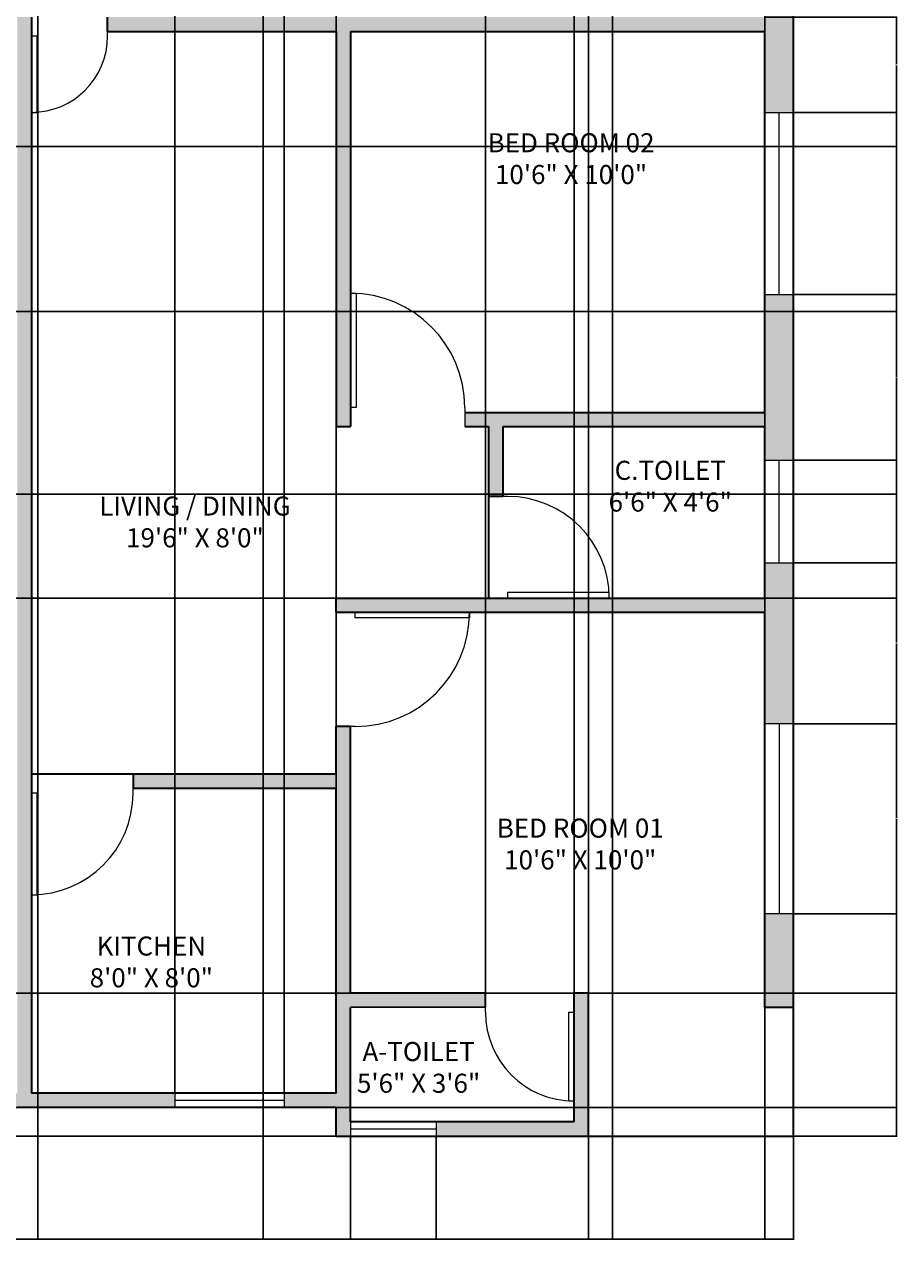
# Model space of a CAD drawing. Units: inches. Extents: x 2510 to 3056, y 673 to 1386.
# Tile 2 of 4: x 2781 to 3056, y 673 to 1056. Entities that reach past the tile are written whole.
import ezdxf

# ---------------------------------------------------------------- set-up
doc = ezdxf.new("R2010")
doc.units = ezdxf.units.IN
for name, color, linetype, lineweight in [('A-ANNO-DIMS', 2, 'Continuous', 18), ('A-AREA-IDEN', 7, 'Continuous', 18), ('A-DOOR', 3, 'Continuous', 18), ('A-GLAZ', 4, 'Continuous', 18), ('A-WALL', 7, 'Continuous', 35), ('A-WALL-PATT', 252, 'Continuous', 13)]:
    doc.layers.add(name, color=color, linetype=linetype, lineweight=lineweight)
doc.styles.get("Standard").update_dxf_attribs({"font": 'arial.ttf'})
doc.dimstyles.get("Standard").update_dxf_attribs({"dimtxt": 0.18, "dimasz": 0.18, "dimexe": 0.18, "dimexo": 0.0625, "dimgap": 0.09, "dimtad": 0, "dimtih": 1, "dimtoh": 1, "dimdec": 4, "dimzin": 0, "dimdsep": 46, "dimtxsty": 'Standard', "dimcen": 0.09, "dimadec": 0, "dimazin": 0, "dimtfac": 1, "dimtdec": 4, "dimtofl": 0, "dimtmove": 0, "dimatfit": 3, "dimfxl": 1, "dimtolj": 1, "dimtzin": 0, "dimarcsym": 0})

# ---------------------------------------------------------------- blocks, each defined once
blk = doc.blocks.new('*U6')
for p, q in [((0, 0), (0, -6)), ((36, 0), (36, -6))]:
    blk.add_line(p, q)
blk.add_lwpolyline([(0, 0), (0, 36), (1.75, 36), (1.75, 0)], close=True)
blk.add_arc((0, 0), 36, 0, 90)
blk = doc.blocks.new('*U7')
for p, q in [((0, 0), (0, 6)), ((24, 0), (24, 6))]:
    blk.add_line(p, q)
blk.add_lwpolyline([(0, 0), (0, -24), (1.75, -24), (1.75, 0)], close=True)
blk.add_arc((0, 0), 24, 270, 0)
blk = doc.blocks.new('*U5')
for p, q in [((0, 0), (0, 6)), ((32, 0), (32, 6))]:
    blk.add_line(p, q)
blk.add_lwpolyline([(0, 0), (0, -32), (1.75, -32), (1.75, 0)], close=True)
blk.add_arc((0, 0), 32, 270, 0)
blk = doc.blocks.new('*U11')
for p, q in [((-36, 0), (-36, 6)), ((0, 0), (0, 6))]:
    blk.add_line(p, q)
blk.add_lwpolyline([(0, 0), (0, -36), (-1.75, -36), (-1.75, 0)], close=True)
blk.add_arc((0, 0), 36, 180, 270)
blk = doc.blocks.new('*U10')
for p, q in [((-28, 0), (-28, 6)), ((0, 0), (0, 6))]:
    blk.add_line(p, q)
blk.add_lwpolyline([(0, 0), (0, -28), (-1.75, -28), (-1.75, 0)], close=True)
blk.add_arc((0, 0), 28, 180, 270)
blk = doc.blocks.new('*D13')
at = {"layer": 'A-ANNO-DIMS', "color": 0, "lineweight": -2, "transparency": 16777216}
for p, q in [((2543.19, 705.52), (2543.19, 672.93)), ((3023.19, 705.52), (3023.19, 672.93)), ((2543.37, 673.11), (2782.9, 673.11)), ((3023.01, 673.11), (2783.48, 673.11))]:
    blk.add_line(p, q, dxfattribs=at)
at = {"layer": 'A-ANNO-DIMS', "color": 0, "transparency": 16777216}
for points in [[(2543.37, 673.14), (2543.37, 673.08), (2543.19, 673.11)], [(3023.01, 673.14), (3023.01, 673.08), (3023.19, 673.11)]]:
    blk.add_solid(points, dxfattribs=at)
at = {"layer": 'Defpoints', "color": 0, "transparency": 16777216}
for p in [(2543.19, 705.59), (3023.19, 705.59), (3023.19, 673.11)]:
    blk.add_point(p, dxfattribs=at)
at = {"layer": 'A-ANNO-DIMS', "color": 0, "transparency": 16777216, "insert": (2783.19, 673.11), "char_height": 0.18, "attachment_point": 5}
blk.add_mtext('\\A1;480', dxfattribs=at)
blk = doc.blocks.new('*D22')
at = {"layer": 'A-ANNO-DIMS', "color": 0, "lineweight": -2, "transparency": 16777216}
for p, q in [((3023.25, 775.63), (3055.85, 775.63)), ((3055.67, 775.45), (3055.67, 740.79)), ((3055.67, 705.77), (3055.67, 740.43)), ((3023.25, 705.59), (3055.85, 705.59))]:
    blk.add_line(p, q, dxfattribs=at)
at = {"layer": 'A-ANNO-DIMS', "color": 0, "transparency": 16777216}
for points in [[(3055.64, 775.45), (3055.7, 775.45), (3055.67, 775.63)], [(3055.64, 705.77), (3055.7, 705.77), (3055.67, 705.59)]]:
    blk.add_solid(points, dxfattribs=at)
at = {"layer": 'Defpoints', "color": 0, "transparency": 16777216}
for p in [(3023.19, 775.63), (3055.67, 775.63), (3023.19, 705.59)]:
    blk.add_point(p, dxfattribs=at)
at = {"layer": 'A-ANNO-DIMS', "color": 0, "transparency": 16777216, "insert": (3055.67, 740.61), "char_height": 0.18, "attachment_point": 5}
blk.add_mtext('\\A1;70.04', dxfattribs=at)
blk = doc.blocks.new('*D23')
at = {"layer": 'A-ANNO-DIMS', "color": 0, "lineweight": -2, "transparency": 16777216}
for p, q in [((3023.25, 835.48), (3055.85, 835.48)), ((3055.67, 835.3), (3055.67, 805.74)), ((3055.67, 775.81), (3055.67, 805.37)), ((3023.25, 775.63), (3055.85, 775.63))]:
    blk.add_line(p, q, dxfattribs=at)
at = {"layer": 'A-ANNO-DIMS', "color": 0, "transparency": 16777216}
for points in [[(3055.64, 835.3), (3055.7, 835.3), (3055.67, 835.48)], [(3055.64, 775.81), (3055.7, 775.81), (3055.67, 775.63)]]:
    blk.add_solid(points, dxfattribs=at)
at = {"layer": 'Defpoints', "color": 0, "transparency": 16777216}
for p in [(3023.19, 835.48), (3055.67, 835.48), (3023.19, 775.63)]:
    blk.add_point(p, dxfattribs=at)
at = {"layer": 'A-ANNO-DIMS', "color": 0, "transparency": 16777216, "insert": (3055.67, 805.56), "char_height": 0.18, "attachment_point": 5}
blk.add_mtext('\\A1;59.85', dxfattribs=at)
blk = doc.blocks.new('*D24')
at = {"layer": 'A-ANNO-DIMS', "color": 0, "lineweight": -2, "transparency": 16777216}
for p, q in [((3023.25, 886.22), (3055.85, 886.22)), ((3055.67, 886.04), (3055.67, 861.03)), ((3055.67, 835.66), (3055.67, 860.67)), ((3023.25, 835.48), (3055.85, 835.48))]:
    blk.add_line(p, q, dxfattribs=at)
at = {"layer": 'A-ANNO-DIMS', "color": 0, "transparency": 16777216}
for points in [[(3055.64, 886.04), (3055.7, 886.04), (3055.67, 886.22)], [(3055.64, 835.66), (3055.7, 835.66), (3055.67, 835.48)]]:
    blk.add_solid(points, dxfattribs=at)
at = {"layer": 'Defpoints', "color": 0, "transparency": 16777216}
for p in [(3023.19, 886.22), (3055.67, 886.22), (3023.19, 835.48)]:
    blk.add_point(p, dxfattribs=at)
at = {"layer": 'A-ANNO-DIMS', "color": 0, "transparency": 16777216, "insert": (3055.67, 860.85), "char_height": 0.18, "attachment_point": 5}
blk.add_mtext('\\A1;50.74', dxfattribs=at)
blk = doc.blocks.new('*D25')
at = {"layer": 'A-ANNO-DIMS', "color": 0, "lineweight": -2, "transparency": 16777216}
for p, q in [((3023.25, 918.54), (3055.85, 918.54)), ((3055.67, 918.36), (3055.67, 902.56)), ((3055.67, 886.4), (3055.67, 902.2)), ((3023.25, 886.22), (3055.85, 886.22))]:
    blk.add_line(p, q, dxfattribs=at)
at = {"layer": 'A-ANNO-DIMS', "color": 0, "transparency": 16777216}
for points in [[(3055.64, 918.36), (3055.7, 918.36), (3055.67, 918.54)], [(3055.64, 886.4), (3055.7, 886.4), (3055.67, 886.22)]]:
    blk.add_solid(points, dxfattribs=at)
at = {"layer": 'Defpoints', "color": 0, "transparency": 16777216}
for p in [(3023.19, 918.54), (3055.67, 918.54), (3023.19, 886.22)]:
    blk.add_point(p, dxfattribs=at)
at = {"layer": 'A-ANNO-DIMS', "color": 0, "transparency": 16777216, "insert": (3055.67, 902.38), "char_height": 0.18, "attachment_point": 5}
blk.add_mtext('\\A1;32.32', dxfattribs=at)
blk = doc.blocks.new('*D26')
at = {"layer": 'A-ANNO-DIMS', "color": 0, "lineweight": -2, "transparency": 16777216}
for p, q in [((3023.25, 970.69), (3055.85, 970.69)), ((3055.67, 970.51), (3055.67, 944.8)), ((3055.67, 918.72), (3055.67, 944.43)), ((3023.25, 918.54), (3055.85, 918.54))]:
    blk.add_line(p, q, dxfattribs=at)
at = {"layer": 'A-ANNO-DIMS', "color": 0, "transparency": 16777216}
for points in [[(3055.64, 970.51), (3055.7, 970.51), (3055.67, 970.69)], [(3055.64, 918.72), (3055.7, 918.72), (3055.67, 918.54)]]:
    blk.add_solid(points, dxfattribs=at)
at = {"layer": 'Defpoints', "color": 0, "transparency": 16777216}
for p in [(3023.19, 970.69), (3055.67, 970.69), (3023.19, 918.54)]:
    blk.add_point(p, dxfattribs=at)
at = {"layer": 'A-ANNO-DIMS', "color": 0, "transparency": 16777216, "insert": (3055.67, 944.62), "char_height": 0.18, "attachment_point": 5}
blk.add_mtext('\\A1;52.16', dxfattribs=at)
blk = doc.blocks.new('*D27')
at = {"layer": 'A-ANNO-DIMS', "color": 0, "lineweight": -2, "transparency": 16777216}
for p, q in [((3023.25, 1028.03), (3055.85, 1028.03)), ((3055.67, 1027.85), (3055.67, 999.55)), ((3055.67, 970.87), (3055.67, 999.18)), ((3023.25, 970.69), (3055.85, 970.69))]:
    blk.add_line(p, q, dxfattribs=at)
at = {"layer": 'A-ANNO-DIMS', "color": 0, "transparency": 16777216}
for points in [[(3055.64, 1027.85), (3055.7, 1027.85), (3055.67, 1028.03)], [(3055.64, 970.87), (3055.7, 970.87), (3055.67, 970.69)]]:
    blk.add_solid(points, dxfattribs=at)
at = {"layer": 'Defpoints', "color": 0, "transparency": 16777216}
for p in [(3023.19, 1028.03), (3055.67, 1028.03), (3023.19, 970.69)]:
    blk.add_point(p, dxfattribs=at)
at = {"layer": 'A-ANNO-DIMS', "color": 0, "transparency": 16777216, "insert": (3055.67, 999.36), "char_height": 0.18, "attachment_point": 5}
blk.add_mtext('\\A1;57.34', dxfattribs=at)
blk = doc.blocks.new('*D28')
at = {"layer": 'A-ANNO-DIMS', "color": 0, "lineweight": -2, "transparency": 16777216}
for p, q in [((3014.25, 1058.09), (3055.85, 1058.09)), ((3055.67, 1057.91), (3055.67, 1043.24)), ((3055.67, 1028.21), (3055.67, 1042.88)), ((3023.25, 1028.03), (3055.85, 1028.03))]:
    blk.add_line(p, q, dxfattribs=at)
at = {"layer": 'A-ANNO-DIMS', "color": 0, "transparency": 16777216}
for points in [[(3055.64, 1057.91), (3055.7, 1057.91), (3055.67, 1058.09)], [(3055.64, 1028.21), (3055.7, 1028.21), (3055.67, 1028.03)]]:
    blk.add_solid(points, dxfattribs=at)
at = {"layer": 'Defpoints', "color": 0, "transparency": 16777216}
for p in [(3014.19, 1058.09), (3055.67, 1058.09), (3023.19, 1028.03)]:
    blk.add_point(p, dxfattribs=at)
at = {"layer": 'A-ANNO-DIMS', "color": 0, "transparency": 16777216, "insert": (3055.67, 1043.06), "char_height": 0.18, "attachment_point": 5}
blk.add_mtext('\\A1;30.053', dxfattribs=at)
blk = doc.blocks.new('*D34')
at = {"layer": 'A-ANNO-DIMS', "color": 0, "lineweight": -2, "transparency": 16777216}
for p, q in [((2552.25, 907.81), (3055.85, 907.81)), ((3055.67, 907.63), (3055.67, 891.63)), ((3055.67, 875.27), (3055.67, 891.27)), ((2552.25, 875.09), (3055.85, 875.09))]:
    blk.add_line(p, q, dxfattribs=at)
at = {"layer": 'A-ANNO-DIMS', "color": 0, "transparency": 16777216}
for points in [[(3055.64, 907.63), (3055.7, 907.63), (3055.67, 907.81)], [(3055.64, 875.27), (3055.7, 875.27), (3055.67, 875.09)]]:
    blk.add_solid(points, dxfattribs=at)
at = {"layer": 'Defpoints', "color": 0, "transparency": 16777216}
for p in [(2552.19, 907.81), (3055.67, 907.81), (2552.19, 875.09)]:
    blk.add_point(p, dxfattribs=at)
at = {"layer": 'A-ANNO-DIMS', "color": 0, "transparency": 16777216, "insert": (3055.67, 891.45), "char_height": 0.18, "attachment_point": 5}
blk.add_mtext('\\A1;32.72', dxfattribs=at)
blk = doc.blocks.new('*D35')
at = {"layer": 'A-ANNO-DIMS', "color": 0, "lineweight": -2, "transparency": 16777216}
for p, q in [((2552.25, 1017.32), (3055.85, 1017.32)), ((3055.67, 1017.14), (3055.67, 991.52)), ((3055.67, 965.53), (3055.67, 991.15)), ((2552.25, 965.35), (3055.85, 965.35))]:
    blk.add_line(p, q, dxfattribs=at)
at = {"layer": 'A-ANNO-DIMS', "color": 0, "transparency": 16777216}
for points in [[(3055.64, 1017.14), (3055.7, 1017.14), (3055.67, 1017.32)], [(3055.64, 965.53), (3055.7, 965.53), (3055.67, 965.35)]]:
    blk.add_solid(points, dxfattribs=at)
at = {"layer": 'Defpoints', "color": 0, "transparency": 16777216}
for p in [(2552.19, 1017.32), (3055.67, 1017.32), (2552.19, 965.35)]:
    blk.add_point(p, dxfattribs=at)
at = {"layer": 'A-ANNO-DIMS', "color": 0, "transparency": 16777216, "insert": (3055.67, 991.34), "char_height": 0.18, "attachment_point": 5}
blk.add_mtext('\\A1;51.97', dxfattribs=at)
blk = doc.blocks.new('*D38')
at = {"layer": 'A-ANNO-DIMS', "color": 0, "lineweight": -2, "transparency": 16777216}
for p, q in [((2856.19, 1106.77), (2856.19, 672.93)), ((2966.19, 1106.77), (2966.19, 672.93)), ((2856.37, 673.11), (2910.91, 673.11)), ((2966.01, 673.11), (2911.47, 673.11))]:
    blk.add_line(p, q, dxfattribs=at)
at = {"layer": 'A-ANNO-DIMS', "color": 0, "transparency": 16777216}
for points in [[(2856.37, 673.14), (2856.37, 673.08), (2856.19, 673.11)], [(2966.01, 673.14), (2966.01, 673.08), (2966.19, 673.11)]]:
    blk.add_solid(points, dxfattribs=at)
at = {"layer": 'Defpoints', "color": 0, "transparency": 16777216}
for p in [(2856.19, 1106.84), (2966.19, 1106.84), (2966.19, 673.11)]:
    blk.add_point(p, dxfattribs=at)
at = {"layer": 'A-ANNO-DIMS', "color": 0, "transparency": 16777216, "insert": (2911.19, 673.11), "char_height": 0.18, "attachment_point": 5}
blk.add_mtext('\\A1;110', dxfattribs=at)
blk = doc.blocks.new('*D39')
at = {"layer": 'A-ANNO-DIMS', "color": 0, "lineweight": -2, "transparency": 16777216}
for p, q in [((2966.19, 1155.52), (2966.19, 672.93)), ((3014.19, 1155.52), (3014.19, 672.93)), ((2966.37, 673.11), (2989.97, 673.11)), ((3014.01, 673.11), (2990.42, 673.11))]:
    blk.add_line(p, q, dxfattribs=at)
at = {"layer": 'A-ANNO-DIMS', "color": 0, "transparency": 16777216}
for points in [[(2966.37, 673.14), (2966.37, 673.08), (2966.19, 673.11)], [(3014.01, 673.14), (3014.01, 673.08), (3014.19, 673.11)]]:
    blk.add_solid(points, dxfattribs=at)
at = {"layer": 'Defpoints', "color": 0, "transparency": 16777216}
for p in [(2966.19, 1155.59), (3014.19, 1155.59), (3014.19, 673.11)]:
    blk.add_point(p, dxfattribs=at)
at = {"layer": 'A-ANNO-DIMS', "color": 0, "transparency": 16777216, "insert": (2990.19, 673.11), "char_height": 0.18, "attachment_point": 5}
blk.add_mtext('\\A1;48', dxfattribs=at)
blk = doc.blocks.new('*D42')
at = {"layer": 'A-ANNO-DIMS', "color": 0, "lineweight": -2, "transparency": 16777216}
for p, q in [((2828.31, 719.15), (2828.31, 1386.25)), ((2862.84, 719.15), (2862.84, 1386.25)), ((2828.49, 1386.07), (2845.18, 1386.07)), ((2862.66, 1386.07), (2845.97, 1386.07))]:
    blk.add_line(p, q, dxfattribs=at)
at = {"layer": 'A-ANNO-DIMS', "color": 0, "transparency": 16777216}
for points in [[(2828.49, 1386.1), (2828.49, 1386.04), (2828.31, 1386.07)], [(2862.66, 1386.1), (2862.66, 1386.04), (2862.84, 1386.07)]]:
    blk.add_solid(points, dxfattribs=at)
at = {"layer": 'Defpoints', "color": 0, "transparency": 16777216}
for p in [(2862.84, 1386.07), (2828.31, 719.09), (2862.84, 719.09)]:
    blk.add_point(p, dxfattribs=at)
at = {"layer": 'A-ANNO-DIMS', "color": 0, "transparency": 16777216, "insert": (2845.57, 1386.07), "char_height": 0.18, "attachment_point": 5}
blk.add_mtext('\\A1;34.53', dxfattribs=at)
blk = doc.blocks.new('*D43')
at = {"layer": 'A-ANNO-DIMS', "color": 0, "lineweight": -2, "transparency": 16777216}
for p, q in [((2862.84, 719.15), (2862.84, 1386.25)), ((2879.19, 719.15), (2879.19, 1386.25)), ((2863.02, 1386.07), (2870.56, 1386.07)), ((2879.01, 1386.07), (2871.47, 1386.07))]:
    blk.add_line(p, q, dxfattribs=at)
at = {"layer": 'A-ANNO-DIMS', "color": 0, "transparency": 16777216}
for points in [[(2863.02, 1386.1), (2863.02, 1386.04), (2862.84, 1386.07)], [(2879.01, 1386.1), (2879.01, 1386.04), (2879.19, 1386.07)]]:
    blk.add_solid(points, dxfattribs=at)
at = {"layer": 'Defpoints', "color": 0, "transparency": 16777216}
for p in [(2879.19, 1386.07), (2862.84, 719.09), (2879.19, 719.09)]:
    blk.add_point(p, dxfattribs=at)
at = {"layer": 'A-ANNO-DIMS', "color": 0, "transparency": 16777216, "insert": (2871.02, 1386.07), "char_height": 0.18, "attachment_point": 5}
blk.add_mtext('\\A1;16.354', dxfattribs=at)
blk = doc.blocks.new('*D46')
at = {"layer": 'A-ANNO-DIMS', "color": 0, "lineweight": -2, "transparency": 16777216}
for p, q in [((2753.19, 1256.02), (2753.19, 672.93)), ((2785.19, 1256.02), (2785.19, 672.93)), ((2753.37, 673.11), (2768.97, 673.11)), ((2785.01, 673.11), (2769.41, 673.11))]:
    blk.add_line(p, q, dxfattribs=at)
at = {"layer": 'A-ANNO-DIMS', "color": 0, "transparency": 16777216}
for points in [[(2753.37, 673.14), (2753.37, 673.08), (2753.19, 673.11)], [(2785.01, 673.14), (2785.01, 673.08), (2785.19, 673.11)]]:
    blk.add_solid(points, dxfattribs=at)
at = {"layer": 'Defpoints', "color": 0, "transparency": 16777216}
for p in [(2753.19, 1256.09), (2785.19, 1256.09), (2785.19, 673.11)]:
    blk.add_point(p, dxfattribs=at)
at = {"layer": 'A-ANNO-DIMS', "color": 0, "transparency": 16777216, "insert": (2769.19, 673.11), "char_height": 0.18, "attachment_point": 5}
blk.add_mtext('\\A1;32', dxfattribs=at)
blk = doc.blocks.new('*D47')
at = {"layer": 'A-ANNO-DIMS', "color": 0, "lineweight": -2, "transparency": 16777216}
for p, q in [((2926.19, 750.65), (2926.19, 1386.25)), ((2954.19, 750.65), (2954.19, 1386.25)), ((2926.37, 1386.07), (2939.97, 1386.07)), ((2954.01, 1386.07), (2940.41, 1386.07))]:
    blk.add_line(p, q, dxfattribs=at)
at = {"layer": 'A-ANNO-DIMS', "color": 0, "transparency": 16777216}
for points in [[(2926.37, 1386.1), (2926.37, 1386.04), (2926.19, 1386.07)], [(2954.01, 1386.1), (2954.01, 1386.04), (2954.19, 1386.07)]]:
    blk.add_solid(points, dxfattribs=at)
at = {"layer": 'Defpoints', "color": 0, "transparency": 16777216}
for p in [(2954.19, 1386.07), (2926.19, 750.59), (2954.19, 750.59)]:
    blk.add_point(p, dxfattribs=at)
at = {"layer": 'A-ANNO-DIMS', "color": 0, "transparency": 16777216, "insert": (2940.19, 1386.07), "char_height": 0.18, "attachment_point": 5}
blk.add_mtext('\\A1;28', dxfattribs=at)
blk = doc.blocks.new('*D48')
at = {"layer": 'A-ANNO-DIMS', "color": 0, "lineweight": -2, "transparency": 16777216}
for p, q in [((2883.69, 705.52), (2883.69, 672.93)), ((2910.68, 705.52), (2910.68, 672.93)), ((2883.87, 673.11), (2896.79, 673.11)), ((2910.5, 673.11), (2897.58, 673.11))]:
    blk.add_line(p, q, dxfattribs=at)
at = {"layer": 'A-ANNO-DIMS', "color": 0, "transparency": 16777216}
for points in [[(2883.87, 673.14), (2883.87, 673.08), (2883.69, 673.11)], [(2910.5, 673.14), (2910.5, 673.08), (2910.68, 673.11)]]:
    blk.add_solid(points, dxfattribs=at)
at = {"layer": 'Defpoints', "color": 0, "transparency": 16777216}
for p in [(2883.69, 705.59), (2910.68, 705.59), (2910.68, 673.11)]:
    blk.add_point(p, dxfattribs=at)
at = {"layer": 'A-ANNO-DIMS', "color": 0, "transparency": 16777216, "insert": (2897.19, 673.11), "char_height": 0.18, "attachment_point": 5}
blk.add_mtext('\\A1;26.99', dxfattribs=at)
blk = doc.blocks.new('*D49')
at = {"layer": 'A-ANNO-DIMS', "color": 0, "lineweight": -2, "transparency": 16777216}
for p, q in [((2910.68, 705.52), (2910.68, 672.93)), ((2958.69, 705.52), (2958.69, 672.93)), ((2910.86, 673.11), (2934.31, 673.11)), ((2958.51, 673.11), (2935.07, 673.11))]:
    blk.add_line(p, q, dxfattribs=at)
at = {"layer": 'A-ANNO-DIMS', "color": 0, "transparency": 16777216}
for points in [[(2910.86, 673.14), (2910.86, 673.08), (2910.68, 673.11)], [(2958.51, 673.14), (2958.51, 673.08), (2958.69, 673.11)]]:
    blk.add_solid(points, dxfattribs=at)
at = {"layer": 'Defpoints', "color": 0, "transparency": 16777216}
for p in [(2910.68, 705.59), (2958.69, 705.59), (2958.69, 673.11)]:
    blk.add_point(p, dxfattribs=at)
at = {"layer": 'A-ANNO-DIMS', "color": 0, "transparency": 16777216, "insert": (2934.69, 673.11), "char_height": 0.18, "attachment_point": 5}
blk.add_mtext('\\A1;48.01', dxfattribs=at)
blk = doc.blocks.new('*D53')
at = {"layer": 'A-ANNO-DIMS', "color": 0, "lineweight": -2, "transparency": 16777216}
for p, q in [((2682.75, 714.59), (3055.85, 714.59)), ((3055.67, 714.41), (3055.67, 710.27)), ((3055.67, 705.77), (3055.67, 709.9)), ((2682.75, 705.59), (3055.85, 705.59))]:
    blk.add_line(p, q, dxfattribs=at)
at = {"layer": 'A-ANNO-DIMS', "color": 0, "transparency": 16777216}
for points in [[(3055.64, 714.41), (3055.7, 714.41), (3055.67, 714.59)], [(3055.64, 705.77), (3055.7, 705.77), (3055.67, 705.59)]]:
    blk.add_solid(points, dxfattribs=at)
at = {"layer": 'Defpoints', "color": 0, "transparency": 16777216}
for p in [(2682.69, 714.59), (3055.67, 714.59), (2682.69, 705.59)]:
    blk.add_point(p, dxfattribs=at)
at = {"layer": 'A-ANNO-DIMS', "color": 0, "transparency": 16777216, "insert": (3055.67, 710.09), "char_height": 0.18, "attachment_point": 5}
blk.add_mtext('\\A1;9', dxfattribs=at)
blk = doc.blocks.new('*D54')
at = {"layer": 'A-ANNO-DIMS', "color": 0, "lineweight": -2, "transparency": 16777216}
for p, q in [((2678.25, 750.59), (3055.85, 750.59)), ((3055.67, 750.41), (3055.67, 732.77)), ((3055.67, 714.77), (3055.67, 732.4)), ((2682.75, 714.59), (3055.85, 714.59))]:
    blk.add_line(p, q, dxfattribs=at)
at = {"layer": 'A-ANNO-DIMS', "color": 0, "transparency": 16777216}
for points in [[(3055.64, 750.41), (3055.7, 750.41), (3055.67, 750.59)], [(3055.64, 714.77), (3055.7, 714.77), (3055.67, 714.59)]]:
    blk.add_solid(points, dxfattribs=at)
at = {"layer": 'Defpoints', "color": 0, "transparency": 16777216}
for p in [(2678.19, 750.59), (3055.67, 750.59), (2682.69, 714.59)]:
    blk.add_point(p, dxfattribs=at)
at = {"layer": 'A-ANNO-DIMS', "color": 0, "transparency": 16777216, "insert": (3055.67, 732.59), "char_height": 0.18, "attachment_point": 5}
blk.add_mtext('\\A1;36', dxfattribs=at)
blk = doc.blocks.new('*D55')
at = {"layer": 'A-ANNO-DIMS', "color": 0, "lineweight": -2, "transparency": 16777216}
for p, q in [((2958.75, 750.59), (3055.85, 750.59)), ((3055.67, 750.41), (3055.67, 728.27)), ((3055.67, 705.77), (3055.67, 727.9)), ((2958.75, 705.59), (3055.85, 705.59))]:
    blk.add_line(p, q, dxfattribs=at)
at = {"layer": 'A-ANNO-DIMS', "color": 0, "transparency": 16777216}
for points in [[(3055.64, 750.41), (3055.7, 750.41), (3055.67, 750.59)], [(3055.64, 705.77), (3055.7, 705.77), (3055.67, 705.59)]]:
    blk.add_solid(points, dxfattribs=at)
at = {"layer": 'Defpoints', "color": 0, "transparency": 16777216}
for p in [(2958.69, 750.59), (3055.67, 750.59), (2958.69, 705.59)]:
    blk.add_point(p, dxfattribs=at)
at = {"layer": 'A-ANNO-DIMS', "color": 0, "transparency": 16777216, "insert": (3055.67, 728.09), "char_height": 0.18, "attachment_point": 5}
blk.add_mtext('\\A1;45', dxfattribs=at)
blk = doc.blocks.new('*D56')
at = {"layer": 'A-ANNO-DIMS', "color": 0, "lineweight": -2, "transparency": 16777216}
for p, q in [((2954.19, 750.65), (2954.19, 1386.25)), ((2958.69, 750.65), (2958.69, 1386.25)), ((2954.37, 1386.07), (2956.18, 1386.07)), ((2958.51, 1386.07), (2956.7, 1386.07))]:
    blk.add_line(p, q, dxfattribs=at)
at = {"layer": 'A-ANNO-DIMS', "color": 0, "transparency": 16777216}
for points in [[(2954.37, 1386.1), (2954.37, 1386.04), (2954.19, 1386.07)], [(2958.51, 1386.1), (2958.51, 1386.04), (2958.69, 1386.07)]]:
    blk.add_solid(points, dxfattribs=at)
at = {"layer": 'Defpoints', "color": 0, "transparency": 16777216}
for p in [(2958.69, 1386.07), (2954.19, 750.59), (2958.69, 750.59)]:
    blk.add_point(p, dxfattribs=at)
at = {"layer": 'A-ANNO-DIMS', "color": 0, "transparency": 16777216, "insert": (2956.44, 1386.07), "char_height": 0.18, "attachment_point": 5}
blk.add_mtext('\\A1;4.5', dxfattribs=at)
blk = doc.blocks.new('*D58')
at = {"layer": 'A-ANNO-DIMS', "color": 0, "lineweight": -2, "transparency": 16777216}
for p, q in [((2958.69, 705.65), (2958.69, 1386.25)), ((3023.19, 705.65), (3023.19, 1386.25)), ((2958.87, 1386.07), (2990.62, 1386.07)), ((3023.01, 1386.07), (2991.27, 1386.07))]:
    blk.add_line(p, q, dxfattribs=at)
at = {"layer": 'A-ANNO-DIMS', "color": 0, "transparency": 16777216}
for points in [[(2958.87, 1386.1), (2958.87, 1386.04), (2958.69, 1386.07)], [(3023.01, 1386.1), (3023.01, 1386.04), (3023.19, 1386.07)]]:
    blk.add_solid(points, dxfattribs=at)
at = {"layer": 'Defpoints', "color": 0, "transparency": 16777216}
for p in [(3023.19, 1386.07), (2958.69, 705.59), (3023.19, 705.59)]:
    blk.add_point(p, dxfattribs=at)
at = {"layer": 'A-ANNO-DIMS', "color": 0, "transparency": 16777216, "insert": (2990.94, 1386.07), "char_height": 0.18, "attachment_point": 5}
blk.add_mtext('\\A1;64.5', dxfattribs=at)

msp = doc.modelspace()

# ---------------------------------------------------------------- hatches: boundary and pattern name
at = {"layer": 'A-WALL-PATT'}
h = msp.add_hatch(color=256, dxfattribs=at)
h.dxf.hatch_style = 1
h.paths.add_polyline_path([(2580.5162, 1353.5862), (2543.1924, 1353.5862), (2543.1924, 1311.5591), (2552.1924, 1311.5591), (2552.1924, 1344.5862), (2580.5162, 1344.5862)])
h.paths.add_polyline_path([(2720.7125, 1353.5862), (2648.0497, 1353.5862), (2648.0497, 1344.5862), (2696.1924, 1344.5862), (2696.1924, 1208.0862), (2700.6924, 1208.0862), (2700.6924, 1256.0862), (2716.6924, 1256.0862), (2716.6924, 1260.5862), (2700.6924, 1260.5862), (2700.6924, 1344.5862), (2720.7125, 1344.5862)])
h.paths.add_polyline_path([(2762.4727, 1353.5862), (2748.6924, 1353.5862), (2748.6924, 1344.5862), (2748.6924, 1256.0862), (2753.1924, 1256.0862), (2753.1924, 1262.0862), (2753.1924, 1294.0862), (2753.1924, 1344.5862), (2762.4727, 1344.5862)])
h.paths.add_polyline_path([(2863.5016, 1353.5862), (2808.6621, 1353.5862), (2808.6621, 1344.5862), (2825.1924, 1344.5862), (2825.1924, 1260.5862), (2785.1924, 1260.5862), (2785.1924, 1256.0862), (2825.1924, 1256.0862), (2825.1924, 1248.5862), (2829.6924, 1248.5862), (2829.6924, 1344.5862), (2863.5016, 1344.5862)])
h.paths.add_polyline_path([(2966.1924, 1353.5862), (2915.7284, 1353.5862), (2915.7284, 1344.5862), (2961.6924, 1344.5862), (2961.6924, 1212.5862), (2897.6924, 1212.5862), (2897.6924, 1208.0862), (2961.6924, 1208.0862), (2961.6924, 1193.4346), (2966.1924, 1193.4346), (2966.1924, 1208.0862)])
h.paths.add_polyline_path([(2660.1924, 1212.5862), (2552.1924, 1212.5862), (2552.1924, 1254.8401), (2543.1924, 1254.8401), (2543.1924, 1168.7504), (2552.1924, 1168.7504), (2552.1924, 1208.0862), (2660.1924, 1208.0862)])
h.paths.add_polyline_path([(3023.1924, 1160.0862), (2966.1924, 1160.0862), (2966.1924, 1165.033), (2961.6924, 1165.033), (2961.6924, 1160.0862), (2865.6924, 1160.0862), (2865.6924, 1212.5862), (2825.1924, 1212.5862), (2825.1924, 1208.0862), (2861.1924, 1208.0862), (2861.1924, 1160.0862), (2750.1527, 1160.0862), (2750.1527, 1155.5862), (2754.6527, 1155.5862), (2966.1924, 1155.5862), (3014.1924, 1155.5862), (3014.1924, 1136.4806), (3023.1924, 1136.4806)])
h.paths.add_polyline_path([(3023.1924, 1090.8839), (3014.1924, 1090.8839), (3014.1924, 1058.0862), (2807.1924, 1058.0862), (2807.1924, 1053.5862), (2879.1924, 1053.5862), (2879.1924, 929.0862), (2883.6924, 929.0862), (2883.6924, 935.0862), (2883.6924, 971.0862), (2883.6924, 1053.5862), (3014.1924, 1053.5862), (3014.1924, 1028.0329), (3023.1924, 1028.0329)])
h.paths.add_polyline_path([(3023.1924, 970.6943), (3014.1924, 970.6943), (3014.1924, 933.5862), (2919.6924, 933.5862), (2919.6924, 929.0862), (2927.1924, 929.0862), (2927.1924, 907.0862), (2931.6924, 907.0862), (2931.6924, 929.0862), (3014.1924, 929.0862), (3014.1924, 918.5377), (3023.1924, 918.5377)])
h.paths.add_polyline_path([(3023.1924, 886.219), (3014.1924, 886.219), (3014.1924, 875.0862), (2927.1924, 875.0862), (2879.1924, 875.0862), (2879.1924, 870.5862), (2885.1924, 870.5862), (2921.1924, 870.5862), (3014.1924, 870.5862), (3014.1924, 835.4806), (3023.1924, 835.4806)])
h.paths.add_polyline_path([(3023.1924, 775.6299), (3014.1924, 775.6299), (3014.1924, 746.0862), (3023.1924, 746.0862)])
h.paths.add_polyline_path([(2958.6924, 750.5862), (2954.1924, 750.5862), (2954.1924, 744.5862), (2954.1924, 716.5862), (2954.1924, 710.0862), (2910.6841, 710.0862), (2910.6841, 705.5862), (2958.6924, 705.5862)])
h.paths.add_polyline_path([(2926.1924, 750.5862), (2883.6924, 750.5862), (2883.6924, 834.5862), (2879.1924, 834.5862), (2879.1924, 819.5862), (2815.1924, 819.5862), (2815.1924, 815.0862), (2879.1924, 815.0862), (2879.1924, 746.0862), (2879.1924, 719.0862), (2862.8388, 719.0862), (2862.8388, 714.5862), (2879.1924, 714.5862), (2879.1924, 705.5862), (2883.6924, 705.5862), (2883.6924, 710.0862), (2883.6924, 746.0862), (2926.1924, 746.1758)])
h.paths.add_polyline_path([(2682.6924, 815.0862), (2746.6924, 815.0862), (2746.6924, 819.5862), (2682.6924, 819.5862), (2682.6924, 834.5862), (2678.1924, 834.5862), (2678.1924, 750.5862), (2639.6924, 750.5862), (2639.6924, 746.0862), (2678.1924, 746.0862), (2678.1924, 710.0862), (2678.1924, 705.5862), (2682.6924, 705.5862), (2682.6924, 714.5862), (2699.7376, 714.5862), (2699.7376, 719.0862), (2682.6924, 719.0862), (2682.6924, 746.0862)])
h.paths.add_polyline_path([(2650.2761, 710.0862), (2607.6924, 710.0862), (2607.6924, 750.5862), (2603.1924, 750.5862), (2603.1924, 705.5862), (2607.6924, 705.5862), (2650.2761, 705.5862)])
h.paths.add_polyline_path([(2552.1924, 777.7158), (2543.1924, 777.7158), (2543.1924, 746.0862), (2552.1924, 746.0862)])
h.paths.add_polyline_path([(2828.3093, 719.0862), (2783.1924, 719.0862), (2783.1924, 815.0862), (2783.1924, 1058.0862), (2778.6924, 1058.0862), (2778.6924, 815.0862), (2778.6924, 719.0862), (2743.8813, 719.0862), (2743.8813, 714.5862), (2778.6924, 714.5862), (2828.3093, 714.5862)])
h.paths.add_polyline_path([(2642.1924, 933.5862), (2552.1924, 933.5862), (2552.1924, 965.3494), (2543.1924, 965.3494), (2543.1924, 907.809), (2552.1924, 907.809), (2552.1924, 929.0862), (2630.1924, 929.0862), (2630.1924, 907.0862), (2634.6924, 907.0862), (2634.6924, 929.0862), (2642.1924, 929.0862)])
h.paths.add_polyline_path([(2682.6924, 875.0862), (2552.1924, 875.0862), (2543.1924, 875.0862), (2543.1924, 832.3664), (2552.1924, 832.3664), (2552.1924, 870.5862), (2634.6924, 870.5862), (2682.6924, 870.5862)])
h.paths.add_polyline_path([(2754.6527, 1119.5862), (2750.1527, 1119.5862), (2750.1527, 1058.0862), (2552.1924, 1058.0862), (2552.1924, 1104.0128), (2543.1924, 1104.0128), (2543.1924, 1017.3235), (2552.1924, 1017.3235), (2552.1924, 1053.5862), (2678.1924, 1053.5862), (2678.1924, 929.0862), (2682.6924, 929.0862), (2682.6924, 1053.5862), (2754.6527, 1053.5862)])

# ---------------------------------------------------------------- linework, layer by layer
at = {"layer": 'A-GLAZ'}
for p, q in [((3014.1924, 1028.0329), (3023.1924, 1028.0329)), ((3018.6924, 970.6943), (3018.6924, 1028.0329)), ((3014.1924, 970.6943), (3023.1924, 970.6943)), ((3014.1924, 918.5377), (3023.1924, 918.5377)), ((3018.6924, 886.219), (3018.6924, 918.5377)), ((3014.1924, 886.219), (3023.1924, 886.219)), ((3023.1924, 835.4806), (3014.1924, 835.4806)), ((3018.6924, 835.4806), (3018.6924, 775.6299)), ((3023.1924, 775.6299), (3014.1924, 775.6299)), ((2828.3093, 719.0862), (2828.3093, 714.5862)), ((2828.3093, 716.8362), (2862.8388, 716.8362)), ((2862.8388, 719.0862), (2862.8388, 714.5862)), ((2883.6924, 710.0862), (2883.6924, 705.5862)), ((2910.6841, 710.0862), (2910.6841, 705.5862)), ((2883.6924, 707.8362), (2910.6841, 707.8362))]:
    msp.add_line(p, q, dxfattribs=at)
at = {"layer": 'A-WALL'}
for p, q in [((3023.1924, 705.5862), (3023.1924, 1160.0862)), ((2783.1924, 1058.0862), (2783.1924, 815.0862)), ((2807.1924, 1053.5862), (2807.1924, 1058.0862)), ((2807.1924, 1053.5862), (2879.1924, 1053.5862)), ((2879.1924, 1053.5862), (2879.1924, 929.0862)), ((2883.6924, 1053.5862), (2883.6924, 929.0862)), ((2883.6924, 1053.5862), (3014.1924, 1053.5862)), ((3014.1924, 933.5862), (3014.1924, 1053.5862)), ((2919.6924, 933.5862), (3014.1924, 933.5862)), ((2879.1924, 929.0862), (2883.6924, 929.0862)), ((2919.6924, 929.0862), (2927.1924, 929.0862)), ((2927.1924, 929.0862), (2927.1924, 875.0862)), ((2931.6924, 929.0862), (2931.6924, 907.0862)), ((2931.6924, 929.0862), (3014.1924, 929.0862)), ((3014.1924, 875.0862), (3014.1924, 929.0862)), ((2931.6924, 907.0862), (2927.1924, 907.0862)), ((2879.1924, 875.0862), (2927.1924, 875.0862)), ((2879.1924, 870.5862), (2879.1924, 875.0862)), ((2927.1924, 875.0862), (3014.1924, 875.0862)), ((2879.1924, 870.5862), (3014.1924, 870.5862)), ((3014.1924, 746.0862), (3014.1924, 870.5862)), ((2883.6924, 834.5862), (2879.1924, 834.5862)), ((2879.1924, 819.5862), (2879.1924, 834.5862)), ((2883.6924, 750.5862), (2883.6924, 834.5862)), ((2879.1924, 819.5862), (2783.1924, 819.5862)), ((2815.1924, 819.5862), (2815.1924, 815.0862)), ((2783.1924, 815.0862), (2783.1924, 719.0862)), ((2879.1924, 815.0862), (2815.1924, 815.0862)), ((2879.1924, 746.0862), (2879.1924, 815.0862)), ((2926.1924, 750.5862), (2883.6924, 750.5862)), ((2926.1924, 746.1758), (2926.1924, 750.5862)), ((2958.6924, 750.5862), (2954.1924, 750.5862)), ((2954.1924, 710.0862), (2954.1924, 750.5862)), ((2958.6924, 705.5862), (2958.6924, 750.5862)), ((2879.1924, 719.0862), (2879.1924, 746.0862)), ((2926.1924, 746.1758), (2883.6924, 746.0862)), ((2883.6924, 710.0862), (2883.6924, 746.0862)), ((3023.1924, 746.0862), (3014.1924, 746.0862)), ((2879.1924, 719.0862), (2783.1924, 719.0862)), ((2879.1924, 714.5862), (2778.6924, 714.5862)), ((2879.1924, 705.5862), (2879.1924, 714.5862)), ((2954.1924, 710.0862), (2883.6924, 710.0862)), ((2879.1924, 705.5862), (3023.1924, 705.5862))]:
    msp.add_line(p, q, dxfattribs=at)

# ---------------------------------------------------------------- block references
at = {"layer": 'A-DOOR'}
for name, p in [('*U7', (2783.1924, 1052.0862)), ('*U6', (2883.6924, 935.0862)), ('*U5', (2783.1924, 813.5862)), ('*U10', (2954.1924, 744.5862))]:
    msp.add_blockref(name, p, dxfattribs=at)
at = {"layer": 'A-DOOR', "rotation": 90}
for name, p in [('*U5', (2933.1924, 875.0862)), ('*U11', (2885.1924, 870.5862))]:
    msp.add_blockref(name, p, dxfattribs=at)

# ---------------------------------------------------------------- texts
at = {"layer": 'A-AREA-IDEN', "char_height": 6, "attachment_point": 1}
for s, width, insert in [('\\pxqc;BED ROOM 02\\P10\'6" X 10\'0"', 59.569763, (2923.3752, 1021.5192)), ('\\pxqc;C.TOILET\\P6\'6" X 4\'6"', 59.569763, (2954.6227, 918.3195)), ('\\pxqc;LIVING / DINING\\P19\'6" X 8\'0"', 74.309254, (2797.5348, 907.0622)), ('\\pxqc;BED ROOM 01\\P10\'6" X 10\'0"', 59.569763, (2926.2696, 805.5866)), ('\\pxqc;KITCHEN\\P8\'0" X 8\'0"', 59.569763, (2791.1689, 768.4431)), ('\\pxqc;A-TOILET\\P5\'6" X 3\'6"', 43.694303, (2883.2981, 735.2118))]:
    msp.add_mtext_dynamic_manual_height_columns(s, width=width, gutter_width=12.5, heights=[0], dxfattribs=dict(at, insert=insert))

# ---------------------------------------------------------------- dimensions: what is measured, and where the dimension line sits
at = {"layer": 'A-ANNO-DIMS'}
for base, p1, p2, override, picture, middle in [((2862.8388, 1386.0667), (2828.3093, 719.0862), (2862.8388, 719.0862), {"dimdec": 2, "dimlfac": 1, "dimrnd": 0, "dimzin": 0, "dimdsep": 46, "dimlunit": 2}, '*D42', (2845.5741, 1386.0667)), ((2879.1924, 1386.0667), (2862.8388, 719.0862), (2879.1924, 719.0862), {"dimdec": 3, "dimlfac": 1, "dimrnd": 0, "dimzin": 0, "dimdsep": 46, "dimlunit": 2}, '*D43', (2871.0156, 1386.0667)), ((2954.1924, 1386.0667), (2926.1924, 750.5862), (2954.1924, 750.5862), {"dimdec": 0, "dimlfac": 1, "dimrnd": 0, "dimzin": 0, "dimdsep": 46, "dimlunit": 2}, '*D47', (2940.1924, 1386.0667)), ((2958.6924, 1386.0667), (2954.1924, 750.5862), (2958.6924, 750.5862), {"dimdec": 1, "dimlfac": 1, "dimrnd": 0, "dimzin": 0, "dimdsep": 46, "dimlunit": 2}, '*D56', (2956.4424, 1386.0667)), ((3023.1924, 1386.0667), (2958.6924, 705.5862), (3023.1924, 705.5862), {"dimdec": 1, "dimlfac": 1, "dimrnd": 0, "dimzin": 0, "dimdsep": 46, "dimlunit": 2}, '*D58', (2990.9424, 1386.0667)), ((2785.1924, 673.1057), (2753.1924, 1256.0862), (2785.1924, 1256.0862), {"dimdec": 0, "dimlfac": 1, "dimrnd": 0, "dimzin": 0, "dimdsep": 46, "dimlunit": 2}, '*D46', (2769.1924, 673.1057)), ((3014.1924, 673.1057), (2966.1924, 1155.5862), (3014.1924, 1155.5862), {"dimdec": 0, "dimlfac": 1, "dimrnd": 0, "dimzin": 0, "dimdsep": 46, "dimlunit": 2}, '*D39', (2990.1924, 673.1057)), ((2966.1924, 673.1057), (2856.1924, 1106.8362), (2966.1924, 1106.8362), {"dimdec": 0, "dimlfac": 1, "dimrnd": 0, "dimzin": 0, "dimdsep": 46, "dimlunit": 2}, '*D38', (2911.1924, 673.1057)), ((3023.1924, 673.1057), (2543.1924, 705.5862), (3023.1924, 705.5862), {"dimdec": 0, "dimlfac": 1, "dimrnd": 0, "dimzin": 0, "dimdsep": 46, "dimlunit": 2}, '*D13', (2783.1924, 673.1057)), ((2910.6841, 673.1057), (2883.6924, 705.5862), (2910.6841, 705.5862), {"dimdec": 2, "dimlfac": 1, "dimrnd": 0, "dimzin": 0, "dimdsep": 46, "dimlunit": 2}, '*D48', (2897.1883, 673.1057)), ((2958.6924, 673.1057), (2910.6841, 705.5862), (2958.6924, 705.5862), {"dimdec": 2, "dimlfac": 1, "dimrnd": 0, "dimzin": 0, "dimdsep": 46, "dimlunit": 2}, '*D49', (2934.6883, 673.1057))]:
    dim = msp.add_linear_dim(base=base, p1=p1, p2=p2, dimstyle='Standard', override=override, dxfattribs=at)
    dim.commit()
    dim.dimension.update_dxf_attribs({"geometry": picture, "text_midpoint": middle})
for base, p1, p2, override, picture, middle in [((3055.6729, 1058.0862), (3023.1924, 1028.0329), (3014.1924, 1058.0862), {"dimdec": 3, "dimlfac": 1, "dimrnd": 0, "dimzin": 0, "dimdsep": 46, "dimlunit": 2}, '*D28', (3055.6729, 1043.0595)), ((3055.6729, 1028.0329), (3023.1924, 970.6943), (3023.1924, 1028.0329), {"dimdec": 2, "dimlfac": 1, "dimrnd": 0, "dimzin": 0, "dimdsep": 46, "dimlunit": 2}, '*D27', (3055.6729, 999.3636)), ((3055.6729, 1017.3235), (2552.1924, 965.3494), (2552.1924, 1017.3235), {"dimdec": 2, "dimlfac": 1, "dimrnd": 0, "dimzin": 0, "dimdsep": 46, "dimlunit": 2}, '*D35', (3055.6729, 991.3364)), ((3055.6729, 970.6943), (3023.1924, 918.5377), (3023.1924, 970.6943), {"dimdec": 2, "dimlfac": 1, "dimrnd": 0, "dimzin": 0, "dimdsep": 46, "dimlunit": 2}, '*D26', (3055.6729, 944.616)), ((3055.6729, 918.5377), (3023.1924, 886.219), (3023.1924, 918.5377), {"dimdec": 2, "dimlfac": 1, "dimrnd": 0, "dimzin": 0, "dimdsep": 46, "dimlunit": 2}, '*D25', (3055.6729, 902.3784)), ((3055.6729, 907.809), (2552.1924, 875.0862), (2552.1924, 907.809), {"dimdec": 2, "dimlfac": 1, "dimrnd": 0, "dimzin": 0, "dimdsep": 46, "dimlunit": 2}, '*D34', (3055.6729, 891.4476)), ((3055.6729, 886.219), (3023.1924, 835.4806), (3023.1924, 886.219), {"dimdec": 2, "dimlfac": 1, "dimrnd": 0, "dimzin": 0, "dimdsep": 46, "dimlunit": 2}, '*D24', (3055.6729, 860.8498)), ((3055.6729, 835.4806), (3023.1924, 775.6299), (3023.1924, 835.4806), {"dimdec": 2, "dimlfac": 1, "dimrnd": 0, "dimzin": 0, "dimdsep": 46, "dimlunit": 2}, '*D23', (3055.6729, 805.5552)), ((3055.6729, 775.6299), (3023.1924, 705.5862), (3023.1924, 775.6299), {"dimdec": 2, "dimlfac": 1, "dimrnd": 0, "dimzin": 0, "dimdsep": 46, "dimlunit": 2}, '*D22', (3055.6729, 740.608)), ((3055.6729, 750.5862), (2682.6924, 714.5862), (2678.1924, 750.5862), {"dimdec": 0, "dimlfac": 1, "dimrnd": 0, "dimzin": 0, "dimdsep": 46, "dimlunit": 2}, '*D54', (3055.6729, 732.5862)), ((3055.6729, 750.5862), (2958.6924, 705.5862), (2958.6924, 750.5862), {"dimdec": 0, "dimlfac": 1, "dimrnd": 0, "dimzin": 0, "dimdsep": 46, "dimlunit": 2}, '*D55', (3055.6729, 728.0862)), ((3055.6729, 714.5862), (2682.6924, 705.5862), (2682.6924, 714.5862), {"dimdec": 0, "dimlfac": 1, "dimrnd": 0, "dimzin": 0, "dimdsep": 46, "dimlunit": 2}, '*D53', (3055.6729, 710.0862))]:
    dim = msp.add_linear_dim(base=base, p1=p1, p2=p2, angle=90, dimstyle='Standard', override=override, dxfattribs=at)
    dim.commit()
    dim.dimension.update_dxf_attribs({"geometry": picture, "text_midpoint": middle})

doc.saveas('drawing.dxf')
